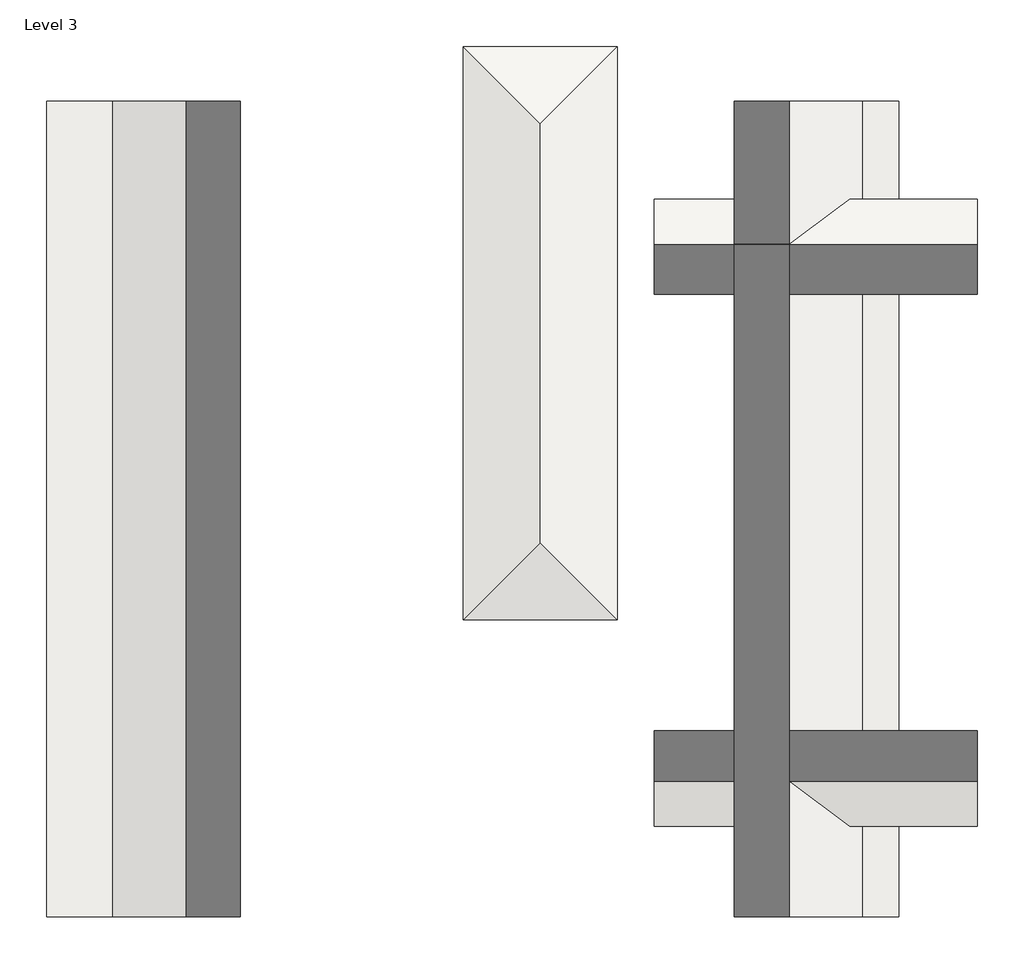
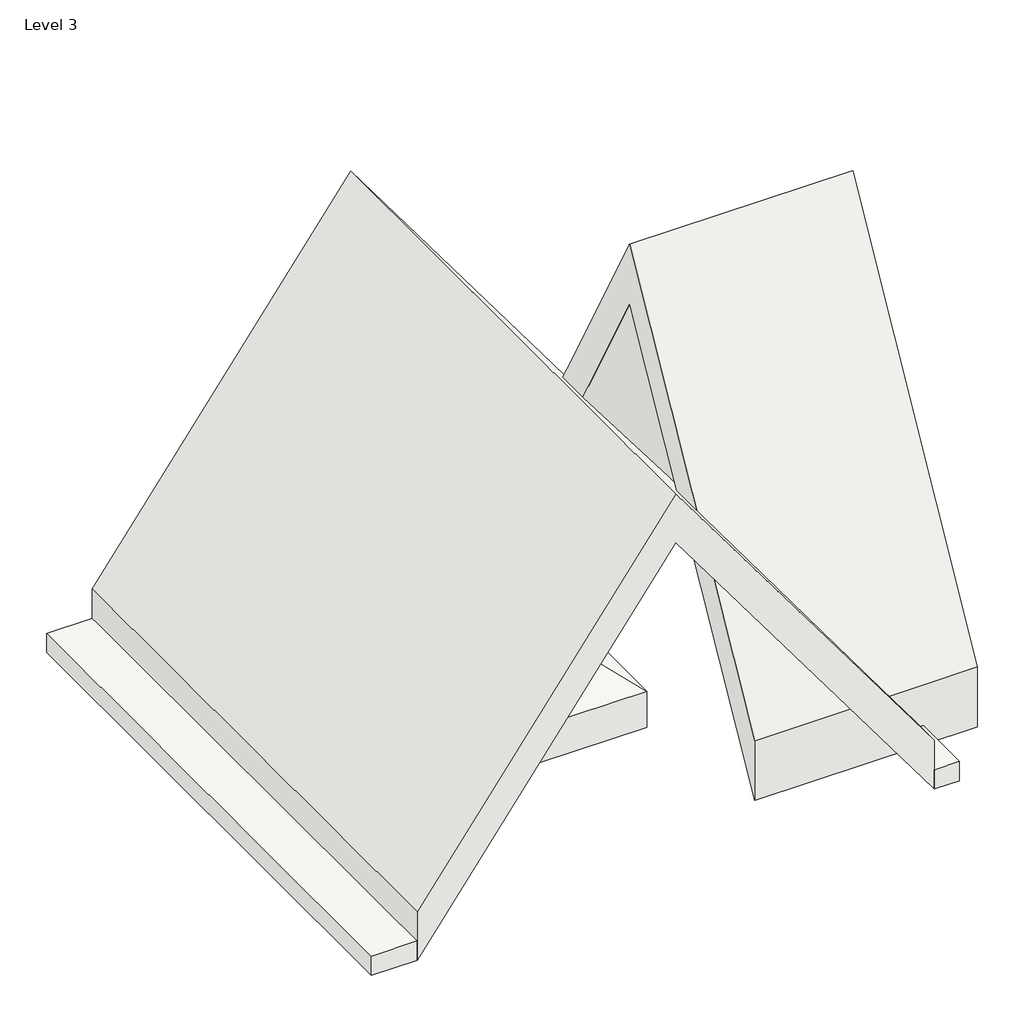
# One storey: 3 roofs, 2 coverings.
"""IFC4 building model written with IfcOpenShell, lengths in millimetres."""

from ifc_helpers import new_model, si_unit, frame, origin, place, context, project, spatial, polyline, outline, extrude, faceted_brep, element, save

model = new_model("IFC4")

# Units and contexts
model_context = context("Model", 3, world=origin())
ifc_project = project(units=[si_unit("LENGTHUNIT", "METRE", prefix="MILLI")], contexts=[model_context])

# Site, building, storey
site = spatial("IfcSite", under=ifc_project)
building = spatial("IfcBuilding", under=site)
storey = spatial("IfcBuildingStorey", under=building, Name="Level 3", Elevation=6096.0)

# Coverings
placement = place(None, origin())
element("IfcCovering", 1, ObjectType="Generic - 8\"", at=placement, inside=storey, context=model_context, shape_type="SweptSolid", body=[
    extrude(outline(polyline([(-4388.456206, -7765.1253823), (-4642.456206, -7765.1253823), (-4642.456206, -2126.3253823), (-4388.456206, -2126.3253823), (-4388.456206, -7765.1253823)])), frame((0.0, 0.0, 6096.0), z_axis=(0.0, 0.0, 1.0), x_axis=(1.0, 0.0, 0.0)), (0.0, 0.0, 1.0), 203.2),
])
element("IfcCovering", 2, ObjectType="Generic - 8\"", at=placement, inside=storey, context=model_context, shape_type="SweptSolid", body=[
    extrude(outline(polyline([(-10281.256206, -7765.1253823), (-10281.256206, -2126.3253823), (-9824.056206, -2126.3253823), (-9824.056206, -7765.1253823), (-10281.256206, -7765.1253823)])), frame((0.0, 0.0, 6096.0), z_axis=(0.0, 0.0, 1.0), x_axis=(1.0, 0.0, 0.0)), (0.0, 0.0, 1.0), 203.2),
])

# Roofs
element("IfcRoof", 3, ObjectType="Generic - 12\"", at=placement, inside=storey, context=model_context, shape_type="SweptSolid", body=[
    extrude(outline(polyline([(6610.2399921, -4642.456206), (10130.7151662, -7233.256206), (6610.2399921, -9824.056206), (6096.0, -9824.056206), (9616.4751741, -7233.256206), (6096.0, -4642.456206), (6610.2399921, -4642.456206)])), frame((0.0, -7765.1253823, 0.0), z_axis=(0.0, 1.0, 0.0), x_axis=(0.0, 0.0, 1.0)), (0.0, 0.0, 1.0), 5638.8),
])
element("IfcRoof", 4, ObjectType="Generic - 12\"", at=placement, inside=storey, context=model_context, shape_type="Brep", body=[
    faceted_brep([(-7400.9236456, -5709.6035369, 6096.0), (-6867.5236456, -5176.2035369, 6496.05), (-6334.1236456, -5709.6035369, 6096.0), (-6867.5236456, -2280.6035369, 6496.05), (-6334.1236456, -1747.2035369, 6096.0), (-7400.9236456, -1747.2035369, 6096.0), (-7400.9236456, -5709.6035369, 6477.0), (-6334.1236456, -5709.6035369, 6477.0), (-6867.5236456, -5176.2035369, 6877.05), (-6334.1236456, -1747.2035369, 6477.0), (-6867.5236456, -2280.6035369, 6877.05), (-7400.9236456, -1747.2035369, 6477.0)], [[[0, 1, 2]], [[2, 1, 3, 4]], [[4, 3, 5]], [[1, 0, 5, 3]], [[6, 7, 8]], [[7, 9, 10, 8]], [[9, 11, 10]], [[6, 8, 10, 11]], [[2, 7, 6, 0]], [[4, 9, 7, 2]], [[5, 11, 9, 4]], [[0, 6, 11, 5]]]),
])
element("IfcRoof", 5, ObjectType="Generic - 12\"", at=placement, inside=storey, context=model_context, shape_type="SweptSolid", body=[
    extrude(outline(polyline([(-7137.4598836, 6729.5110837), (-4970.1849805, 10678.4429132), (-2802.9100774, 6729.5110837), (-2802.9100774, 6096.0), (-4970.1849805, 10044.9318295), (-7137.4598836, 6096.0), (-7137.4598836, 6729.5110837)])), frame((-6078.3046146, 0.0, 0.0), z_axis=(1.0, 0.0, 0.0), x_axis=(0.0, 1.0, 0.0)), (0.0, 0.0, 1.0), 2233.2745552),
])

save(model, "model.ifc")

# Revit data of these elements
# Type "Generic - 8\""
#   built-in parameter 1002203 = 1 (stored number, unit not read)
#   built-in parameter 1002202 = 1 (stored number, unit not read)
#   Layers, outside or top first: 0' - 8" no material (function 1)
# Type "Generic - 12\""
#   Assembly Code = "B1020"
#   Layers, outside or top first: 1' - 0" no material (function 1)
# Elements 1, 2 (IfcCovering, "Generic - 8\"")
#   Height Offset From Level = 0' - 0"
#   Phase Created = New Construction
#   Materials on its faces: "Default Roof"
# Element 3 (IfcRoof, "Generic - 12\"")
#   built-in parameter 1001705 = 33.2373 (stored number, unit not read)
#   built-in parameter 1001710 = 33615
#   Phase Created = New Construction
#   Materials on its faces: "Default Roof"
# Element 4 (IfcRoof, "Generic - 12\"")
#   built-in parameter 1001705 = 22.5625 (stored number, unit not read)
#   built-in parameter 1001710 = 33615
#   Phase Created = New Construction
#   Materials on its faces: "Default Roof"
# Element 5 (IfcRoof, "Generic - 12\"")
#   built-in parameter 1001705 = 35.0343 (stored number, unit not read)
#   built-in parameter 1001710 = 33615
#   Phase Created = New Construction
#   Materials on its faces: "Default Roof"
# Materials
#   "Default Roof": colour RGB 88 101 114, transparency 0
